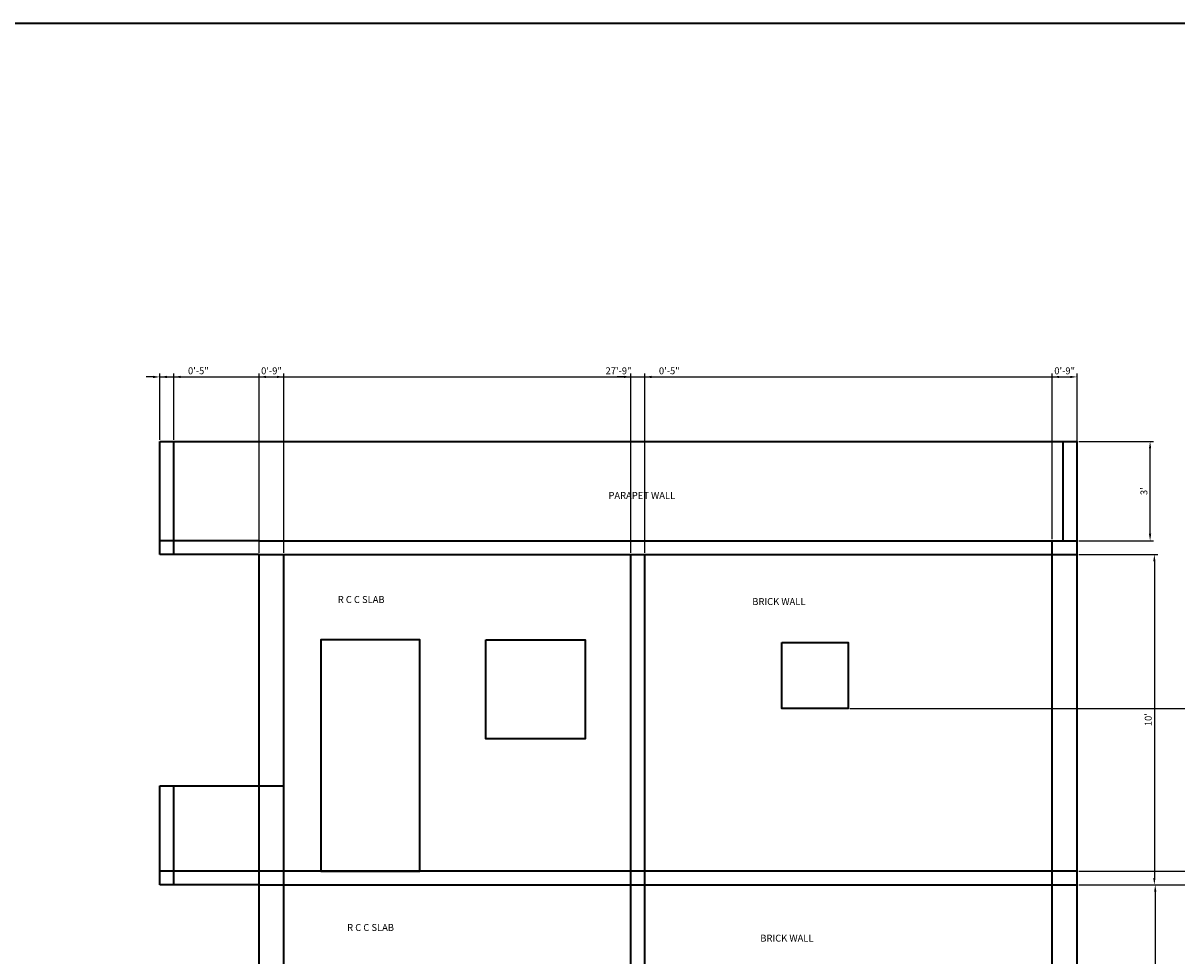
# Model space of a CAD drawing. Units: inches. Extents: x 2020 to 7901, y 1581 to 3943.
# Tile 16 of 17: x 2875 to 3294, y 2728 to 3067. Entities that reach past the tile are written whole.
import ezdxf

# ---------------------------------------------------------------- set-up
doc = ezdxf.new("R2010")
doc.units = ezdxf.units.IN
for name, color, linetype, lineweight in [('A-ANNO-DIMS', 2, 'Continuous', 18), ('A-ANNO-TEXT', 7, 'Continuous', 18), ('A-ANNO-TTLB', 7, 'Continuous', 35), ('A-SECT', 7, 'Continuous', 35)]:
    doc.layers.add(name, color=color, linetype=linetype, lineweight=lineweight)
doc.styles.get("Standard").update_dxf_attribs({"font": 'arial.ttf'})
doc.dimstyles.new('ISO-25', dxfattribs={"dimtxt": 2.5, "dimasz": 2.5, "dimexe": 1.25, "dimexo": 0.625, "dimtad": 1, "dimdec": 1, "dimlunit": 3, "dimtxsty": 'Standard', "dimcen": 2.5, "dimadec": 0, "dimazin": 0, "dimtfac": 1, "dimtdec": 1, "dimtmove": 0, "dimatfit": 3, "dimfxl": 1, "dimarcsym": 0})

# ---------------------------------------------------------------- blocks, each defined once
blk = doc.blocks.new('*D17')
at = {"layer": 'A-ANNO-DIMS', "color": 0, "lineweight": -2, "transparency": 16777216}
for p, q in [((3257.93, 2874.21), (3286.63, 2874.21)), ((3285.38, 2871.71), (3285.38, 2756.71)), ((3257.93, 2754.21), (3286.63, 2754.21))]:
    blk.add_line(p, q, dxfattribs=at)
at = {"layer": 'A-ANNO-DIMS', "color": 0, "transparency": 16777216}
for points in [[(3284.97, 2871.71), (3285.8, 2871.71), (3285.38, 2874.21)], [(3284.97, 2756.71), (3285.8, 2756.71), (3285.38, 2754.21)]]:
    blk.add_solid(points, dxfattribs=at)
at = {"layer": 'DEFPOINTS', "color": 0, "transparency": 16777216}
for p in [(3257.31, 2874.21), (3257.31, 2754.21), (3285.38, 2754.21)]:
    blk.add_point(p, dxfattribs=at)
at = {"layer": 'A-ANNO-DIMS', "color": 0, "transparency": 16777216, "insert": (3283.48, 2814.21), "char_height": 2.5, "attachment_point": 5, "rotation": 90}
blk.add_mtext("10'", dxfattribs=at)
blk = doc.blocks.new('*D18')
at = {"layer": 'A-ANNO-DIMS', "color": 0, "lineweight": -2, "transparency": 16777216}
for p, q in [((3272.91, 2754.21), (3286.95, 2754.21)), ((3285.7, 2751.71), (3285.7, 2636.71)), ((3257.93, 2634.21), (3286.95, 2634.21))]:
    blk.add_line(p, q, dxfattribs=at)
at = {"layer": 'A-ANNO-DIMS', "color": 0, "transparency": 16777216}
for points in [[(3285.28, 2751.71), (3286.12, 2751.71), (3285.7, 2754.21)], [(3285.28, 2636.71), (3286.12, 2636.71), (3285.7, 2634.21)]]:
    blk.add_solid(points, dxfattribs=at)
at = {"layer": 'DEFPOINTS', "color": 0, "transparency": 16777216}
for p in [(3272.28, 2754.21), (3257.31, 2634.21), (3285.7, 2634.21)]:
    blk.add_point(p, dxfattribs=at)
at = {"layer": 'A-ANNO-DIMS', "color": 0, "transparency": 16777216, "insert": (3283.8, 2694.21), "char_height": 2.5, "attachment_point": 5, "rotation": 90}
blk.add_mtext("10'", dxfattribs=at)
blk = doc.blocks.new('*D21')
at = {"layer": 'A-ANNO-DIMS', "color": 0, "lineweight": -2, "transparency": 16777216}
for p, q in [((3257.93, 2915.21), (3285.08, 2915.21)), ((3283.83, 2881.71), (3283.83, 2912.71)), ((3257.93, 2879.21), (3285.08, 2879.21))]:
    blk.add_line(p, q, dxfattribs=at)
at = {"layer": 'A-ANNO-DIMS', "color": 0, "transparency": 16777216}
for points in [[(3283.41, 2912.71), (3284.24, 2912.71), (3283.83, 2915.21)], [(3283.41, 2881.71), (3284.24, 2881.71), (3283.83, 2879.21)]]:
    blk.add_solid(points, dxfattribs=at)
at = {"layer": 'DEFPOINTS', "color": 0, "transparency": 16777216}
for p in [(3257.31, 2915.21), (3283.83, 2915.21), (3257.31, 2879.21)]:
    blk.add_point(p, dxfattribs=at)
at = {"layer": 'A-ANNO-DIMS', "color": 0, "transparency": 16777216, "insert": (3281.92, 2897.21), "char_height": 2.5, "attachment_point": 5, "rotation": 90}
blk.add_mtext("3'", dxfattribs=at)
blk = doc.blocks.new('*D81')
at = {"layer": 'A-ANNO-DIMS', "color": 0, "lineweight": -2, "transparency": 16777216}
for p, q in [((2924.31, 2915.83), (2924.31, 2939.96)), ((2926.81, 2938.71), (3254.81, 2938.71)), ((3257.31, 2915.83), (3257.31, 2939.96))]:
    blk.add_line(p, q, dxfattribs=at)
at = {"layer": 'A-ANNO-DIMS', "color": 0, "transparency": 16777216}
for points in [[(2926.81, 2939.12), (2926.81, 2938.29), (2924.31, 2938.71)], [(3254.81, 2939.12), (3254.81, 2938.29), (3257.31, 2938.71)]]:
    blk.add_solid(points, dxfattribs=at)
at = {"layer": 'DEFPOINTS', "color": 0, "transparency": 16777216}
for p in [(3257.31, 2938.71), (2924.31, 2915.21), (3257.31, 2915.21)]:
    blk.add_point(p, dxfattribs=at)
at = {"layer": 'A-ANNO-DIMS', "color": 0, "transparency": 16777216, "insert": (3090.81, 2940.61), "char_height": 2.5, "attachment_point": 5}
blk.add_mtext('27\'-9"', dxfattribs=at)
blk = doc.blocks.new('*D159')
at = {"layer": 'A-ANNO-DIMS', "color": 0, "lineweight": -2, "transparency": 16777216}
for p, q in [((3329.38, 2761.71), (3329.38, 2772.1)), ((3257.93, 2759.21), (3330.63, 2759.21)), ((3329.38, 2754.21), (3329.38, 2759.21)), ((3257.93, 2754.21), (3330.63, 2754.21)), ((3329.38, 2751.71), (3329.38, 2749.21))]:
    blk.add_line(p, q, dxfattribs=at)
at = {"layer": 'A-ANNO-DIMS', "color": 0, "transparency": 16777216}
for points in [[(3328.96, 2761.71), (3329.8, 2761.71), (3329.38, 2759.21)], [(3328.96, 2751.71), (3329.8, 2751.71), (3329.38, 2754.21)]]:
    blk.add_solid(points, dxfattribs=at)
at = {"layer": 'DEFPOINTS', "color": 0, "transparency": 16777216}
for p in [(3257.31, 2759.21), (3329.38, 2759.21), (3257.31, 2754.21)]:
    blk.add_point(p, dxfattribs=at)
at = {"layer": 'A-ANNO-DIMS', "color": 0, "transparency": 16777216, "insert": (3327.48, 2768.16), "char_height": 2.5, "attachment_point": 5, "rotation": 90}
blk.add_mtext('0\'-5"', dxfattribs=at)
blk = doc.blocks.new('*D161')
at = {"layer": 'A-ANNO-DIMS', "color": 0, "lineweight": -2, "transparency": 16777216}
for p, q in [((2960.31, 2874.83), (2960.31, 2939.96)), ((2962.81, 2938.71), (2966.81, 2938.71)), ((2969.31, 2874.83), (2969.31, 2939.96))]:
    blk.add_line(p, q, dxfattribs=at)
at = {"layer": 'A-ANNO-DIMS', "color": 0, "transparency": 16777216}
for points in [[(2962.81, 2939.12), (2962.81, 2938.29), (2960.31, 2938.71)], [(2966.81, 2939.12), (2966.81, 2938.29), (2969.31, 2938.71)]]:
    blk.add_solid(points, dxfattribs=at)
at = {"layer": 'DEFPOINTS', "color": 0, "transparency": 16777216}
for p in [(2969.31, 2938.71), (2960.31, 2874.21), (2969.31, 2874.21)]:
    blk.add_point(p, dxfattribs=at)
at = {"layer": 'A-ANNO-DIMS', "color": 0, "transparency": 16777216, "insert": (2964.81, 2940.61), "char_height": 2.5, "attachment_point": 5}
blk.add_mtext('0\'-9"', dxfattribs=at)
blk = doc.blocks.new('*D162')
at = {"layer": 'A-ANNO-DIMS', "color": 0, "lineweight": -2, "transparency": 16777216}
for p, q in [((3092.81, 2938.71), (3090.31, 2938.71)), ((3095.31, 2874.83), (3095.31, 2939.96)), ((3095.31, 2938.71), (3100.31, 2938.71)), ((3100.31, 2874.83), (3100.31, 2939.96)), ((3102.81, 2938.71), (3113.2, 2938.71))]:
    blk.add_line(p, q, dxfattribs=at)
at = {"layer": 'A-ANNO-DIMS', "color": 0, "transparency": 16777216}
for points in [[(3092.81, 2939.12), (3092.81, 2938.29), (3095.31, 2938.71)], [(3102.81, 2939.12), (3102.81, 2938.29), (3100.31, 2938.71)]]:
    blk.add_solid(points, dxfattribs=at)
at = {"layer": 'DEFPOINTS', "color": 0, "transparency": 16777216}
for p in [(3100.31, 2938.71), (3095.31, 2874.21), (3100.31, 2874.21)]:
    blk.add_point(p, dxfattribs=at)
at = {"layer": 'A-ANNO-DIMS', "color": 0, "transparency": 16777216, "insert": (3109.25, 2940.61), "char_height": 2.5, "attachment_point": 5}
blk.add_mtext('0\'-5"', dxfattribs=at)
blk = doc.blocks.new('*D163')
at = {"layer": 'A-ANNO-DIMS', "color": 0, "lineweight": -2, "transparency": 16777216}
for p, q in [((3248.31, 2879.83), (3248.31, 2939.96)), ((3250.81, 2938.71), (3254.81, 2938.71)), ((3257.31, 2874.83), (3257.31, 2939.96))]:
    blk.add_line(p, q, dxfattribs=at)
at = {"layer": 'A-ANNO-DIMS', "color": 0, "transparency": 16777216}
for points in [[(3250.81, 2939.12), (3250.81, 2938.29), (3248.31, 2938.71)], [(3254.81, 2939.12), (3254.81, 2938.29), (3257.31, 2938.71)]]:
    blk.add_solid(points, dxfattribs=at)
at = {"layer": 'DEFPOINTS', "color": 0, "transparency": 16777216}
for p in [(3257.31, 2938.71), (3248.31, 2879.21), (3257.31, 2874.21)]:
    blk.add_point(p, dxfattribs=at)
at = {"layer": 'A-ANNO-DIMS', "color": 0, "transparency": 16777216, "insert": (3252.81, 2940.61), "char_height": 2.5, "attachment_point": 5}
blk.add_mtext('0\'-9"', dxfattribs=at)
blk = doc.blocks.new('*D164')
at = {"layer": 'A-ANNO-DIMS', "color": 0, "lineweight": -2, "transparency": 16777216}
for p, q in [((2921.81, 2938.71), (2919.31, 2938.71)), ((2924.31, 2915.83), (2924.31, 2939.96)), ((2924.31, 2938.71), (2929.31, 2938.71)), ((2929.31, 2915.83), (2929.31, 2939.96)), ((2931.81, 2938.71), (2942.2, 2938.71))]:
    blk.add_line(p, q, dxfattribs=at)
at = {"layer": 'A-ANNO-DIMS', "color": 0, "transparency": 16777216}
for points in [[(2921.81, 2939.12), (2921.81, 2938.29), (2924.31, 2938.71)], [(2931.81, 2939.12), (2931.81, 2938.29), (2929.31, 2938.71)]]:
    blk.add_solid(points, dxfattribs=at)
at = {"layer": 'DEFPOINTS', "color": 0, "transparency": 16777216}
for p in [(2929.31, 2938.71), (2924.31, 2915.21), (2929.31, 2915.21)]:
    blk.add_point(p, dxfattribs=at)
at = {"layer": 'A-ANNO-DIMS', "color": 0, "transparency": 16777216, "insert": (2938.25, 2940.61), "char_height": 2.5, "attachment_point": 5}
blk.add_mtext('0\'-5"', dxfattribs=at)
blk = doc.blocks.new('*D166')
at = {"layer": 'A-ANNO-DIMS', "color": 0, "lineweight": -2, "transparency": 16777216}
for p, q in [((3174.76, 2818.27), (3330.63, 2818.27)), ((3329.38, 2815.77), (3329.38, 2761.71)), ((3257.93, 2759.21), (3330.63, 2759.21))]:
    blk.add_line(p, q, dxfattribs=at)
at = {"layer": 'A-ANNO-DIMS', "color": 0, "transparency": 16777216}
for points in [[(3328.96, 2815.77), (3329.8, 2815.77), (3329.38, 2818.27)], [(3328.96, 2761.71), (3329.8, 2761.71), (3329.38, 2759.21)]]:
    blk.add_solid(points, dxfattribs=at)
at = {"layer": 'DEFPOINTS', "color": 0, "transparency": 16777216}
for p in [(3174.14, 2818.27), (3257.31, 2759.21), (3329.38, 2759.21)]:
    blk.add_point(p, dxfattribs=at)
at = {"layer": 'A-ANNO-DIMS', "color": 0, "transparency": 16777216, "insert": (3327.5, 2788.74), "char_height": 2.5, "attachment_point": 5, "rotation": 90}
blk.add_mtext('4\'-11"', dxfattribs=at)

msp = doc.modelspace()

# ---------------------------------------------------------------- linework, layer by layer
at = {"layer": 'A-ANNO-TTLB'}
msp.add_lwpolyline([(2019.8, 3067.25), (4199.03, 3067.25), (4199.03, 1580.73), (2019.8, 1580.73)], close=True, dxfattribs=at)
at = {"layer": 'A-SECT'}
for p, q in [((2924.31, 2874.21), (2924.31, 2915.21)), ((2924.31, 2915.21), (2960.31, 2915.21)), ((2929.31, 2874.21), (2929.31, 2915.21)), ((2960.31, 2915.21), (3257.31, 2915.21)), ((3252.31, 2879.21), (3252.31, 2915.21)), ((3257.31, 2491.21), (3257.31, 2915.21)), ((2960.31, 2879.21), (2924.31, 2879.21)), ((2960.31, 2879.21), (3257.31, 2879.21)), ((3248.31, 2491.21), (3248.31, 2879.21)), ((2960.31, 2874.21), (2924.31, 2874.21)), ((2960.31, 2874.21), (3257.31, 2874.21)), ((2960.31, 2491.21), (2960.31, 2874.21)), ((2969.31, 2491.21), (2969.31, 2874.21)), ((3095.31, 2514.21), (3095.31, 2874.21)), ((3100.31, 2514.21), (3100.31, 2874.21)), ((2924.31, 2754.21), (2924.31, 2790.21)), ((2924.31, 2790.21), (2969.31, 2790.21)), ((2929.31, 2754.21), (2929.31, 2790.21)), ((2960.31, 2759.21), (2924.31, 2759.21)), ((3257.31, 2759.21), (2960.31, 2759.21)), ((2960.31, 2754.21), (2924.31, 2754.21)), ((2960.31, 2754.21), (3257.31, 2754.21))]:
    msp.add_line(p, q, dxfattribs=at)
for points in [[(2982.68, 2759.21), (3018.68, 2759.21), (3018.68, 2843.21), (2982.68, 2843.21)], [(3042.68, 2843.21), (3078.68, 2843.21), (3078.68, 2807.21), (3042.68, 2807.21)], [(3150.14, 2842.27), (3174.14, 2842.27), (3174.14, 2818.27), (3150.14, 2818.27)]]:
    msp.add_lwpolyline(points, close=True, dxfattribs=at)

# ---------------------------------------------------------------- texts
at = {"layer": 'A-ANNO-TEXT', "char_height": 2.5, "attachment_point": 1}
for s, width, insert in [('PARAPET WALL', 128.2364, (3087.16, 2896.89)), ('R C C SLAB', 53.7463, (2988.87, 2859.1)), ('BRICK WALL', 42.8811, (3139.37, 2858.36)), ('R C C SLAB', 54.6308, (2992.28, 2739.95)), ('BRICK WALL', 36.0211, (3142.3, 2736.08))]:
    msp.add_mtext_dynamic_manual_height_columns(s, width=width, gutter_width=12.5, heights=[0], dxfattribs=dict(at, insert=insert))

# ---------------------------------------------------------------- dimensions: what is measured, and where the dimension line sits
at = {"layer": 'A-ANNO-DIMS'}
for base, p1, p2, picture, middle in [((2929.31, 2938.71), (2924.31, 2915.21), (2929.31, 2915.21), '*D164', (2938.25, 2940.61)), ((3257.31, 2938.71), (2924.31, 2915.21), (3257.31, 2915.21), '*D81', (3090.81, 2940.61)), ((2969.31, 2938.71), (2960.31, 2874.21), (2969.31, 2874.21), '*D161', (2964.81, 2940.61)), ((3100.31, 2938.71), (3095.31, 2874.21), (3100.31, 2874.21), '*D162', (3109.25, 2940.61)), ((3257.31, 2938.71), (3248.31, 2879.21), (3257.31, 2874.21), '*D163', (3252.81, 2940.61))]:
    dim = msp.add_linear_dim(base=base, p1=p1, p2=p2, dimstyle='ISO-25', override={"dimdec": 1, "dimlfac": 1, "dimrnd": 0, "dimzin": 1, "dimdsep": 46, "dimlunit": 4, "dimfrac": 2}, dxfattribs=at)
    dim.commit()
    dim.dimension.update_dxf_attribs({"geometry": picture, "text_midpoint": middle})
for base, p1, p2, override, picture, middle in [((3283.83, 2915.21), (3257.31, 2879.21), (3257.31, 2915.21), {"dimclrd": 0, "dimclre": 0, "dimclrt": 0}, '*D21', (3281.92, 2897.21)), ((3285.38, 2754.21), (3257.31, 2874.21), (3257.31, 2754.21), {"dimclrd": 0, "dimclre": 0, "dimclrt": 0}, '*D17', (3283.48, 2814.21)), ((3329.38, 2759.21), (3174.14, 2818.27), (3257.31, 2759.21), {"dimdec": 1, "dimlfac": 1, "dimrnd": 0, "dimzin": 1, "dimdsep": 46, "dimlunit": 4, "dimfrac": 2}, '*D166', (3327.5, 2788.74)), ((3329.38, 2759.21), (3257.31, 2754.21), (3257.31, 2759.21), {"dimdec": 1, "dimlfac": 1, "dimrnd": 0, "dimzin": 1, "dimdsep": 46, "dimlunit": 4, "dimfrac": 2}, '*D159', (3327.48, 2768.16)), ((3285.7, 2634.21), (3272.28, 2754.21), (3257.31, 2634.21), {"dimclrd": 0, "dimclre": 0, "dimclrt": 0}, '*D18', (3283.8, 2694.21))]:
    dim = msp.add_linear_dim(base=base, p1=p1, p2=p2, angle=90, dimstyle='ISO-25', override=override, dxfattribs=at)
    dim.commit()
    dim.dimension.update_dxf_attribs({"geometry": picture, "text_midpoint": middle})

doc.saveas('drawing.dxf')
